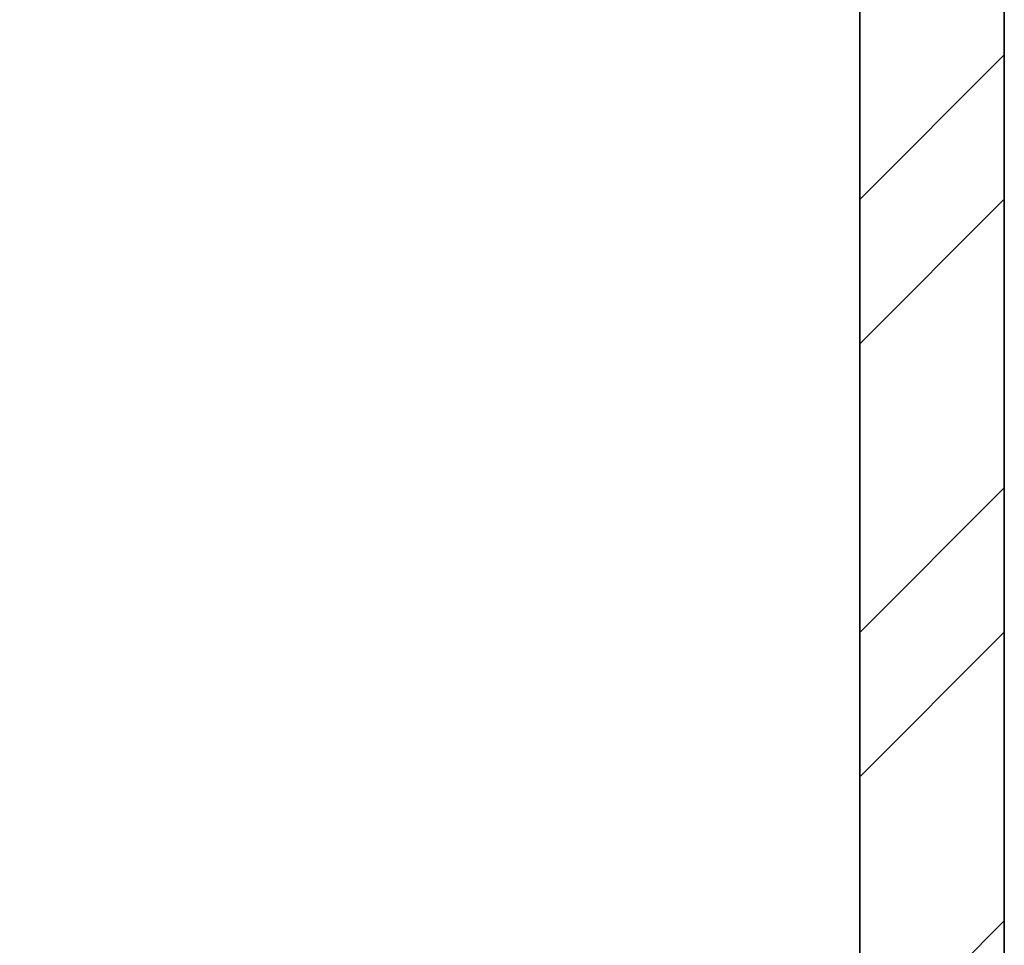
# Model space of a CAD drawing. Units: inches. Extents: x 1885 to 2748, y 783 to 2421.
# Tile 102 of 117: x 2588 to 2618, y 1850 to 1879. Entities that reach past the tile are written whole.
import ezdxf

# ---------------------------------------------------------------- set-up
doc = ezdxf.new("R2010")
doc.units = ezdxf.units.IN
doc.layers.add('A-WALL', color=7, linetype='Continuous', lineweight=35)
doc.layers.add('A-WALL-PATT', color=85, linetype='Continuous', lineweight=13, true_color=0x58ba48)

msp = doc.modelspace()

# ---------------------------------------------------------------- hatches: boundary and pattern name
at = {"layer": 'A-WALL-PATT'}
h = msp.add_hatch(dxfattribs=at)
h.set_pattern_fill('ANSI32', color=256)
h.paths.add_polyline_path([(2007.772, 2318.006), (1980.774, 2318.006), (1980.774, 2281.215), (1985.274, 2281.215), (1985.274, 2313.506), (2007.772, 2313.506), (2007.772, 2315.756)])
h.paths.add_polyline_path([(2094.324, 2318.006), (2067.772, 2318.006), (2067.772, 2313.506), (2094.324, 2313.506), (2094.324, 2315.756)])
h.paths.add_polyline_path([(2131.367, 2315.756), (2131.367, 2318.006), (2131.189, 2318.006), (2112.609, 2318.006), (2112.609, 2313.506), (2117.274, 2313.506), (2117.274, 2255.201), (2121.774, 2255.201), (2121.774, 2313.506), (2131.367, 2313.506)])
h.paths.add_polyline_path([(2190.512, 2318.006), (2155.367, 2318.006), (2155.367, 2313.506), (2169.774, 2313.506), (2169.774, 2229.506), (2121.774, 2229.506), (2121.774, 2233.451), (2119.524, 2233.451), (2117.274, 2233.451), (2117.274, 2201.101), (2121.774, 2201.101), (2121.774, 2225.006), (2169.774, 2225.006), (2169.774, 2165.006), (2306.274, 2165.006), (2306.274, 2066.006), (2310.774, 2066.006), (2344.274, 2066.006), (2486.274, 2066.006), (2486.274, 1886.006), (2483.02, 1886.006), (2483.02, 1881.506), (2486.274, 1881.506), (2486.274, 1880.678), (2490.774, 1880.678), (2490.774, 2070.506), (2344.274, 2070.506), (2310.774, 2070.506), (2310.774, 2165.006), (2310.774, 2173.636), (2308.524, 2173.636), (2306.274, 2173.636), (2306.274, 2169.506), (2174.274, 2169.506), (2174.274, 2313.506), (2190.512, 2313.506), (2190.512, 2315.756)])
h.paths.add_polyline_path([(1985.274, 2221.215), (1980.774, 2221.215), (1980.774, 2165.006), (1992.774, 2165.006), (1992.774, 2141.927), (1997.274, 2141.927), (1997.274, 2165.006), (2117.274, 2165.006), (2117.274, 2163.126), (2121.774, 2163.126), (2121.774, 2172.734), (2119.524, 2172.734), (2117.274, 2172.734), (2117.274, 2169.506), (1985.274, 2169.506)])
h.paths.add_polyline_path([(1997.274, 2105.927), (1992.774, 2105.927), (1992.774, 2070.506), (2016.774, 2070.506), (2016.774, 2059.123), (2019.024, 2059.123), (2021.274, 2059.123), (2021.274, 2070.506), (2117.274, 2070.506), (2117.274, 2022.506), (2114.423, 2022.506), (2114.423, 2018.006), (2123.627, 2018.006), (2123.627, 2020.256), (2123.627, 2022.506), (2121.774, 2022.506), (2121.774, 2142.587), (2119.524, 2142.587), (2117.274, 2142.587), (2117.274, 2075.006), (1997.274, 2075.006)])
h.paths.add_polyline_path([(2092.029, 2020.256), (2092.029, 2022.506), (2021.274, 2022.506), (2021.274, 2035.123), (2016.774, 2035.123), (2016.774, 2018.006), (2016.774, 1978.784), (2021.274, 1978.784), (2021.274, 2018.006), (2092.029, 2018.006)])
h.paths.add_polyline_path([(2260.938, 2022.506), (2153.105, 2022.506), (2153.105, 2020.256), (2153.105, 2018.006), (2155.274, 2018.006), (2155.274, 1886.006), (2107.629, 1886.006), (2107.629, 1881.506), (2182.911, 1881.506), (2182.911, 1883.756), (2182.911, 1886.006), (2159.774, 1886.006), (2159.774, 2018.006), (2260.938, 2018.006), (2260.938, 2020.256)])
h.paths.add_polyline_path([(2047.629, 1883.756), (2047.629, 1886.006), (2021.274, 1886.006), (2021.274, 1918.784), (2019.024, 1918.784), (2016.774, 1918.784), (2016.774, 1881.506), (2047.629, 1881.506)])
h.paths.add_polyline_path([(2306.361, 1883.756), (2306.361, 1886.006), (2296.274, 1886.006), (2296.274, 1982.006), (2316.535, 1982.006), (2316.535, 1984.256), (2316.535, 1986.506), (2296.274, 1986.506), (2296.274, 2022.506), (2289.276, 2022.506), (2289.276, 2018.006), (2291.774, 2018.006), (2291.774, 1886.006), (2242.911, 1886.006), (2242.911, 1881.506), (2306.361, 1881.506)], flags=17)
h.paths.add_polyline_path([(1985.274, 1843.006), (2021.6, 1843.006), (2021.534, 1845.441), (2021.477, 1847.506), (1980.774, 1847.506), (1980.774, 1809.446), (1985.274, 1809.446)])
h.paths.add_polyline_path([(2131.482, 1845.256), (2131.482, 1847.506), (2081.534, 1847.506), (2081.534, 1843.006), (2117.274, 1843.006), (2117.274, 1784.147), (2119.524, 1784.147), (2121.774, 1784.147), (2121.774, 1843.006), (2131.482, 1843.006)])
h.paths.add_polyline_path([(2203.886, 1847.506), (2155.482, 1847.506), (2155.482, 1843.006), (2169.774, 1843.006), (2169.774, 1759.006), (2121.774, 1759.006), (2121.774, 1761.457), (2117.274, 1761.457), (2117.274, 1730.429), (2121.774, 1730.429), (2121.774, 1754.506), (2177.421, 1754.506), (2177.421, 1756.756), (2177.421, 1759.006), (2174.274, 1759.006), (2174.274, 1843.006), (2203.886, 1843.006)])
h.paths.add_polyline_path([(2335.554, 1845.256), (2335.554, 1847.506), (2239.886, 1847.506), (2239.886, 1843.006), (2306.274, 1843.006), (2306.274, 1759.006), (2199.486, 1759.006), (2199.486, 1754.506), (2310.774, 1754.506), (2310.774, 1843.006), (2335.554, 1843.006)])
h.paths.add_polyline_path([(2348.774, 2022.506), (2344.274, 2022.506), (2344.274, 1986.506), (2341.681, 1986.506), (2341.681, 1982.006), (2344.274, 1982.006), (2344.274, 1886.006), (2330.361, 1886.006), (2330.361, 1881.506), (2361.627, 1881.506), (2361.627, 1883.756), (2361.627, 1886.006), (2348.774, 1886.006)], flags=17)
h.paths.add_polyline_path([(2283.251, 2315.756), (2283.251, 2318.006), (2238.512, 2318.006), (2238.512, 2313.506), (2283.251, 2313.506)], flags=17)
h.paths.add_polyline_path([(2363.274, 2348.006), (2388.677, 2348.006), (2388.677, 2350.256), (2388.677, 2352.506), (2358.774, 2352.506), (2358.774, 2348.006), (2358.774, 2318.006), (2344.481, 2318.006), (2344.481, 2313.506), (2358.774, 2313.506), (2358.774, 2229.506), (2310.774, 2229.506), (2310.774, 2231.952), (2306.274, 2231.952), (2306.274, 2205.611), (2310.774, 2205.611), (2310.774, 2225.006), (2358.774, 2225.006), (2358.774, 2211.506), (2452.329, 2211.506), (2452.329, 2213.756), (2452.329, 2216.006), (2363.274, 2216.006), (2363.274, 2318.006)])
h.paths.add_polyline_path([(2310.774, 2313.506), (2320.481, 2313.506), (2320.481, 2315.756), (2320.481, 2318.006), (2302.728, 2318.006), (2302.728, 2313.506), (2306.274, 2313.506), (2306.274, 2251.076), (2310.774, 2251.076)], flags=17)
h.paths.add_polyline_path([(2490.774, 2352.506), (2486.274, 2352.506), (2448.677, 2352.506), (2448.677, 2348.006), (2486.274, 2348.006), (2486.274, 2318.006), (2486.274, 2216.006), (2481.78, 2216.006), (2481.78, 2211.506), (2486.274, 2211.506), (2486.274, 2165.006), (2493.289, 2165.006), (2493.289, 2167.256), (2493.289, 2169.506), (2490.774, 2169.506), (2490.774, 2313.506), (2494.429, 2313.506), (2494.429, 2318.006), (2490.774, 2318.006)])
h.paths.add_polyline_path([(2534.653, 2318.006), (2515.691, 2318.006), (2515.691, 2313.506), (2534.653, 2313.506), (2534.653, 2315.756)])
h.paths.add_polyline_path([(2618.274, 2318.006), (2594.653, 2318.006), (2594.653, 2313.506), (2613.774, 2313.506), (2613.774, 2281.706), (2618.274, 2281.706)])
h.paths.add_polyline_path([(2618.274, 2221.706), (2613.774, 2221.706), (2613.774, 2169.506), (2554.019, 2169.506), (2554.019, 2165.006), (2613.774, 2165.006), (2613.774, 2152.878), (2618.274, 2152.878)])
h.paths.add_polyline_path([(2618.274, 2128.878), (2616.024, 2128.878), (2613.774, 2128.878), (2613.774, 2117.006), (2529.774, 2117.006), (2529.774, 2165.006), (2532.848, 2165.006), (2532.848, 2169.506), (2522.867, 2169.506), (2522.867, 2165.006), (2525.274, 2165.006), (2525.274, 2117.006), (2525.274, 2112.506), (2525.274, 2108.576), (2529.774, 2108.576), (2529.774, 2112.506), (2613.774, 2112.506), (2613.774, 2080.19), (2618.274, 2080.19)])
h.paths.add_polyline_path([(2618.274, 2044.19), (2616.024, 2044.19), (2613.774, 2044.19), (2613.774, 2015.506), (2529.774, 2015.506), (2529.774, 2088.582), (2527.524, 2088.582), (2525.274, 2088.582), (2525.274, 2011.006), (2613.774, 2011.006), (2613.774, 1956.755), (2618.274, 1956.755)])
h.paths.add_polyline_path([(2618.274, 1881.506), (2618.274, 1896.755), (2613.774, 1896.755), (2613.774, 1881.506), (2613.774, 1847.506), (2592.715, 1847.506), (2592.715, 1843.006), (2613.774, 1843.006), (2613.774, 1765.006), (2613.774, 1760.506), (2609.621, 1760.506), (2609.621, 1756.006), (2613.774, 1756.006), (2613.774, 1660.006), (2608.544, 1660.006), (2608.544, 1655.506), (2613.774, 1655.506), (2613.774, 1508.158), (2618.274, 1508.158)])
h.paths.add_polyline_path([(2565.774, 1843.006), (2568.997, 1843.006), (2568.997, 1847.506), (2490.774, 1847.506), (2490.774, 1849.7), (2488.524, 1849.7), (2486.274, 1849.7), (2486.274, 1847.506), (2477.274, 1847.506), (2477.274, 1838.506), (2477.274, 1821.493), (2486.274, 1821.493), (2486.274, 1838.506), (2561.274, 1838.506), (2561.274, 1765.006), (2486.274, 1765.006), (2486.274, 1786.157), (2477.274, 1786.157), (2477.274, 1765.006), (2477.274, 1756.006), (2486.274, 1756.006), (2565.774, 1756.006), (2585.621, 1756.006), (2585.621, 1758.256), (2585.621, 1760.506), (2565.774, 1760.506), (2565.774, 1765.006)])
h.paths.add_polyline_path([(2486.274, 1651.006), (2561.274, 1651.006), (2561.274, 1567.006), (2486.274, 1567.006), (2486.274, 1591.321), (2477.274, 1591.321), (2477.274, 1567.006), (2477.274, 1558.006), (2477.274, 1555.439), (2481.774, 1555.439), (2481.774, 1558.006), (2568.653, 1558.006), (2568.653, 1560.256), (2568.653, 1562.506), (2565.774, 1562.506), (2565.774, 1655.506), (2584.544, 1655.506), (2584.544, 1657.756), (2584.544, 1660.006), (2565.774, 1660.006), (2486.274, 1660.006), (2477.274, 1660.006), (2477.274, 1651.006), (2477.274, 1632.989), (2486.274, 1632.989)])
h.paths.add_polyline_path([(2449.967, 1883.756), (2449.967, 1886.006), (2421.627, 1886.006), (2421.627, 1881.506), (2449.967, 1881.506)], flags=17)
h.paths.add_polyline_path([(2447.274, 1847.506), (2395.554, 1847.506), (2395.554, 1843.006), (2442.774, 1843.006), (2442.774, 1809.27), (2447.274, 1809.27)])
h.paths.add_polyline_path([(1985.274, 1749.446), (1980.774, 1749.446), (1980.774, 1694.504), (1985.274, 1694.504), (1985.274, 1694.506), (1986.897, 1694.506), (1986.897, 1697.78), (1986.897, 1699.006), (1985.274, 1699.006)])
h.paths.add_polyline_path([(2152.774, 1699.006), (2121.774, 1699.006), (2121.774, 1703.668), (2119.524, 1703.668), (2117.274, 1703.668), (2117.274, 1699.006), (2009.219, 1699.006), (2009.219, 1694.506), (2148.274, 1694.506), (2148.274, 1692.631), (2152.774, 1692.631)])
h.paths.add_polyline_path([(2016.274, 1694.506), (2011.774, 1694.506), (2011.774, 1558.006), (2040.806, 1558.006), (2040.806, 1560.256), (2040.806, 1562.506), (2016.274, 1562.506)])
h.paths.add_polyline_path([(2152.774, 1663.017), (2150.524, 1663.017), (2148.274, 1663.017), (2148.274, 1562.506), (2100.806, 1562.506), (2100.806, 1558.006), (2165.119, 1558.006), (2165.119, 1560.256), (2165.119, 1562.506), (2152.774, 1562.506), (2152.774, 1610.506), (2224.774, 1610.506), (2224.774, 1607.99), (2229.274, 1607.99), (2229.274, 1615.006), (2152.774, 1615.006)])
h.paths.add_polyline_path([(2238.613, 1560.256), (2238.613, 1562.506), (2229.274, 1562.506), (2229.274, 1588.756), (2227.024, 1588.763), (2224.774, 1588.771), (2224.774, 1562.506), (2189.119, 1562.506), (2189.119, 1558.006), (2238.613, 1558.006)])
h.paths.add_polyline_path([(2336.024, 1560.256), (2336.024, 1562.506), (2310.774, 1562.506), (2310.774, 1656.347), (2308.524, 1656.347), (2306.274, 1656.347), (2306.274, 1562.506), (2286.613, 1562.506), (2286.613, 1558.006), (2336.024, 1558.006)])
h.paths.add_polyline_path([(2447.274, 1690.968), (2445.024, 1690.968), (2442.774, 1690.968), (2442.774, 1687.006), (2306.274, 1687.006), (2306.274, 1680.75), (2310.774, 1680.75), (2310.774, 1682.506), (2442.774, 1682.506), (2442.774, 1562.506), (2396.024, 1562.506), (2396.024, 1558.006), (2447.274, 1558.006)])
h.paths.add_polyline_path([(2447.274, 1749.27), (2445.024, 1749.27), (2442.774, 1749.27), (2442.774, 1717.232), (2447.274, 1717.232)])
h.paths.add_polyline_path([(2044.674, 1521.756), (2044.674, 1524.006), (2007.274, 1524.006), (2007.274, 1503.49), (2009.524, 1503.49), (2011.774, 1503.49), (2011.774, 1519.506), (2044.674, 1519.506)])
h.paths.add_polyline_path([(2177.969, 1521.756), (2177.969, 1524.006), (2104.674, 1524.006), (2104.674, 1519.506), (2145.774, 1519.506), (2145.774, 1387.506), (2143.37, 1387.506), (2143.37, 1383.006), (2251.585, 1383.006), (2251.585, 1385.256), (2251.585, 1387.506), (2150.274, 1387.506), (2150.274, 1519.506), (2177.969, 1519.506)])
h.paths.add_polyline_path([(2298.704, 1524.006), (2237.969, 1524.006), (2237.969, 1519.506), (2282.274, 1519.506), (2282.274, 1387.506), (2279.683, 1387.506), (2279.683, 1383.006), (2286.774, 1383.006), (2286.774, 1419.006), (2312.451, 1419.006), (2312.451, 1421.256), (2312.451, 1423.506), (2286.774, 1423.506), (2286.774, 1519.506), (2298.704, 1519.506), (2298.704, 1521.722)], flags=17)
h.paths.add_polyline_path([(2361.897, 1521.756), (2361.897, 1524.006), (2322.704, 1524.006), (2322.704, 1519.506), (2334.774, 1519.506), (2334.774, 1423.506), (2331.93, 1423.506), (2331.93, 1419.006), (2334.774, 1419.006), (2334.774, 1387.506), (2334.774, 1383.228), (2339.274, 1383.228), (2339.274, 1387.506), (2339.274, 1519.506), (2361.897, 1519.506)], flags=17)
h.paths.add_polyline_path([(2447.274, 1521.756), (2447.274, 1524.006), (2421.897, 1524.006), (2421.897, 1519.506), (2447.274, 1519.506)], flags=17)
h.paths.add_polyline_path([(2481.774, 1529.6), (2479.524, 1529.6), (2477.274, 1529.6), (2477.274, 1524.006), (2474.489, 1524.006), (2474.489, 1519.506), (2477.274, 1519.506), (2477.274, 1334.506), (2296.774, 1334.506), (2296.774, 1240.506), (2160.274, 1240.506), (2160.274, 1180.506), (2112.274, 1180.506), (2112.274, 1207.692), (2110.024, 1207.692), (2107.774, 1207.692), (2107.774, 1171.609), (2112.274, 1171.609), (2112.274, 1176.006), (2160.274, 1176.006), (2160.274, 1092.006), (2144.221, 1092.006), (2144.221, 1087.506), (2189.497, 1087.506), (2189.497, 1089.756), (2189.497, 1092.006), (2164.774, 1092.006), (2164.774, 1236.006), (2296.774, 1236.006), (2296.774, 1231.912), (2301.274, 1231.912), (2301.274, 1330.006), (2481.774, 1330.006), (2481.774, 1387.506)])
h.paths.add_polyline_path([(2618.274, 1448.158), (2613.774, 1448.158), (2613.774, 1382.506), (2529.774, 1382.506), (2525.274, 1382.506), (2525.274, 1307.062), (2529.774, 1307.062), (2529.774, 1378.006), (2613.774, 1378.006), (2613.774, 1354.988), (2618.274, 1354.988)])
h.paths.add_polyline_path([(2618.274, 1318.988), (2613.774, 1318.988), (2613.774, 1281.006), (2529.774, 1281.006), (2529.774, 1283.786), (2527.524, 1283.786), (2525.274, 1283.786), (2525.274, 1228.506), (2516.794, 1228.506), (2516.794, 1224.006), (2533.484, 1224.006), (2533.484, 1226.256), (2533.484, 1228.506), (2529.774, 1228.506), (2529.774, 1276.506), (2613.774, 1276.506), (2613.774, 1266.02), (2618.274, 1266.02)])
h.paths.add_polyline_path([(2618.274, 1134.964), (2613.774, 1134.964), (2613.774, 1092.006), (2594.545, 1092.006), (2594.545, 1087.506), (2618.274, 1087.506)])
h.paths.add_polyline_path([(2534.545, 1092.006), (2509.765, 1092.006), (2509.765, 1087.506), (2534.545, 1087.506), (2534.545, 1089.756)])
h.paths.add_polyline_path([(2481.274, 1224.006), (2484.117, 1224.006), (2484.117, 1226.256), (2484.117, 1228.506), (2476.774, 1228.506), (2476.774, 1198.506), (2471.61, 1198.506), (2471.61, 1194.006), (2476.774, 1194.006), (2476.774, 1062.006), (2436.894, 1062.006), (2436.894, 1057.506), (2476.774, 1057.506), (2481.274, 1057.506), (2481.274, 1062.006), (2481.274, 1087.506), (2485.354, 1087.506), (2485.354, 1089.756), (2485.354, 1092.006), (2481.274, 1092.006), (2481.274, 1117.506)])
h.paths.add_polyline_path([(2439.898, 1198.506), (2349.274, 1198.506), (2349.274, 1194.006), (2349.274, 1180.506), (2301.274, 1180.506), (2301.274, 1201.896), (2299.024, 1201.896), (2296.774, 1201.896), (2296.774, 1172.335), (2299.024, 1172.335), (2301.274, 1172.335), (2301.274, 1176.006), (2349.274, 1176.006), (2349.274, 1092.006), (2334.452, 1092.006), (2334.452, 1087.506), (2349.274, 1087.506), (2349.274, 1057.506), (2353.774, 1057.506), (2376.894, 1057.506), (2376.894, 1059.756), (2376.894, 1062.006), (2353.774, 1062.006), (2353.774, 1087.506), (2353.774, 1180.506), (2353.774, 1194.006), (2439.898, 1194.006), (2439.898, 1196.256)])
h.paths.add_polyline_path([(2270.596, 1089.756), (2270.596, 1092.006), (2249.497, 1092.006), (2249.497, 1087.506), (2270.596, 1087.506)], flags=17)
h.paths.add_polyline_path([(2310.452, 1092.006), (2301.274, 1092.006), (2301.274, 1153.292), (2296.774, 1153.292), (2296.774, 1092.006), (2293.786, 1092.006), (2293.786, 1087.506), (2310.452, 1087.506), (2310.452, 1089.756)], flags=17)
h.paths.add_polyline_path([(2112.274, 1150.328), (2110.024, 1150.328), (2107.774, 1150.328), (2107.774, 1092.006), (2104.465, 1092.006), (2104.465, 1087.506), (2120.221, 1087.506), (2120.221, 1089.756), (2120.221, 1092.006), (2112.274, 1092.006)])
h.paths.add_polyline_path([(2082.172, 1092.006), (2058.144, 1092.006), (2058.144, 1087.506), (2082.172, 1087.506), (2082.172, 1089.756)])
h.paths.add_polyline_path([(1975.774, 1145.638), (1971.274, 1145.638), (1971.274, 1087.506), (1980.774, 1087.506), (1998.144, 1087.506), (1998.144, 1089.756), (1998.144, 1092.006), (1985.274, 1092.006), (1975.774, 1092.006)])
h.paths.add_polyline_path([(2112.274, 1244.385), (2110.024, 1244.385), (2107.774, 1244.385), (2107.774, 1240.506), (1992.274, 1240.506), (1992.274, 1271.008), (1987.774, 1271.008), (1987.774, 1240.506), (1980.774, 1240.506), (1975.774, 1240.506), (1971.274, 1240.506), (1971.274, 1205.638), (1975.774, 1205.638), (1975.774, 1236.006), (2107.774, 1236.006), (2107.774, 1233.444), (2112.274, 1233.444), (2112.274, 1236.006)])
h.paths.add_polyline_path([(2112.274, 1383.006), (2114.783, 1383.006), (2114.783, 1385.256), (2114.783, 1387.506), (2102.476, 1387.506), (2102.476, 1383.006), (2107.774, 1383.006), (2107.774, 1335.006), (2011.774, 1335.006), (2011.774, 1349.939), (2007.274, 1349.939), (2007.274, 1335.006), (1987.774, 1335.006), (1987.774, 1330.506), (1987.774, 1307.008), (1992.274, 1307.008), (1992.274, 1330.506), (2007.274, 1330.506), (2107.774, 1330.506), (2107.774, 1264.711), (2112.274, 1264.711)])
h.paths.add_polyline_path([(2077.857, 1387.506), (2011.774, 1387.506), (2011.774, 1390.036), (2009.524, 1390.036), (2007.274, 1390.036), (2007.274, 1373.939), (2011.774, 1373.939), (2011.774, 1383.006), (2077.857, 1383.006)])
h.paths.add_polyline_path([(2011.774, 1443.49), (2007.274, 1443.49), (2007.274, 1410.248), (2011.774, 1410.248)])

# ---------------------------------------------------------------- linework, layer by layer
at = {"layer": 'A-WALL'}
for p, q in [((2613.774, 1847.506), (2613.774, 1881.506)), ((2618.274, 1881.506), (2618.274, 1508.158))]:
    msp.add_line(p, q, dxfattribs=at)

doc.saveas('drawing.dxf')
